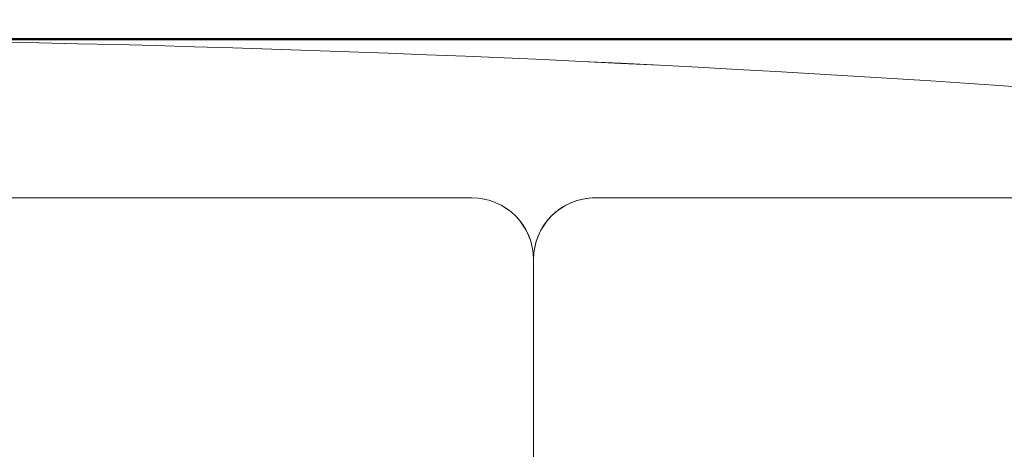
# Model space of a CAD drawing. Units: inches. Extents: x -466983 to 1020, y 324 to 318697.
# Tile 83 of 97: x 650.41 to 662.97, y 948.71 to 954.19. Entities that reach past the tile are written whole.
import ezdxf

# ---------------------------------------------------------------- set-up
doc = ezdxf.new("R2010")
doc.units = ezdxf.units.IN
doc.header["$MEASUREMENT"] = 0
for name, color, linetype, lineweight in [('A-FLOR-PATT', 252, 'Continuous', 13), ('A-FURN', 8, 'Continuous', 18), ('A-WALL', 7, 'Continuous', 50)]:
    doc.layers.add(name, color=color, linetype=linetype, lineweight=lineweight)

# ---------------------------------------------------------------- blocks, each defined once
blk = doc.blocks.new('L Shaped Sofa')
at = {"ltscale": 2}
for p, q in [((2394.712, 728.35), (2394.712, 734.219)), ((2393.28, 726.917), (2377.232, 726.917)), ((2430.914, 726.917), (2396.145, 726.917)), ((2475.263, 723.229), (2377.232, 723.229))]:
    blk.add_line(p, q, dxfattribs=at)
for centre, radius, start, end in [((2393.28, 728.35), 1.433, 270, 0), ((2396.145, 728.35), 1.433, 180, 270), ((2416.36, 1205.029), 481.82, 262.88673, 276.63201)]:
    blk.add_arc(centre, radius, start, end, dxfattribs=at)

msp = doc.modelspace()

# ---------------------------------------------------------------- hatches: boundary and pattern name
at = {"layer": 'A-FLOR-PATT', "transparency": 33554572}
h = msp.add_hatch(dxfattribs=at)
h.set_pattern_fill('ANSI37', color=256, scale=30)
h.set_pattern_definition([(45, (-1212.4137, -290.035), (-2.6516504, 2.6516504), []), (135, (-1212.4137, -290.035), (-2.6516504, -2.6516504), [])])
h.paths.add_polyline_path([(901.806, 1075.938), (900.614, 1075.938), (900.614, 1065.386), (899.391, 1065.386), (898.091, 1065.386), (892.836, 1058.71, -0.258377), (892.188, 1058.351), (879.985, 1058.351, -0.20177), (879.438, 1058.581), (874.081, 1065.386), (872.781, 1065.386), (871.558, 1065.386), (871.558, 1075.938), (813.806, 1075.938), (813.806, 1044.792), (832.395, 1044.792, -0.394795), (848.66, 1028.536), (848.66, 1009.938), (901.806, 1009.938), (901.806, 1015.938), (901.306, 1015.938), (871.306, 1015.938), (871.306, 1017.25), (871.334, 1017.25, -0.401453), (901.306, 1045.938), (901.806, 1045.938)])
edge = h.paths.add_edge_path(flags=16)
edge.add_line((847.773, 1068.949), (847.773, 1073.709))
edge.add_arc((849.227, 1073.709), 1.454, 90, 180, ccw=False)
edge.add_line((849.227, 1075.163), (864.492, 1075.163))
edge.add_arc((864.492, 1073.709), 1.454, 0, 90, ccw=False)
edge.add_line((865.946, 1073.709), (865.946, 1069.004))
edge.add_arc((832.645, 1068.976), 33.301, -20.6123, 0.0472, ccw=False)
edge.add_ellipse((856.859, 1058.48), major_axis=(0, 10.213), ratio=0.685919, start_angle=100.0088, end_angle=259.9912, ccw=False)
edge.add_arc((881.074, 1068.976), 33.301, 180.0472, 200.6123, ccw=False)
h.paths.add_polyline_path([(853.146, 1066.482), (853.146, 1066.453), (853.146, 1066.453, 0.433107), (852.917, 1066.685), (852.917, 1066.453), (853.146, 1066.453), (853.146, 1066.482), (853.088, 1066.612, 0.697939), (852.7, 1066.453), (852.7, 1066.453), (852.7, 1066.482), (852.917, 1067.001), (852.917, 1066.685, -0.396254)], flags=0)
h.paths.add_polyline_path([(861.019, 1066.482), (861.019, 1066.453), (861.019, 1066.453, 0.416404), (860.802, 1066.685), (860.802, 1066.453), (861.019, 1066.453), (861.019, 1066.482), (860.967, 1066.605, 0.713344), (860.573, 1066.453), (860.573, 1066.453), (860.573, 1066.482), (860.802, 1067.001), (860.802, 1066.685, -0.379973)], flags=0)
edge = h.paths.add_edge_path(flags=0)
edge.add_spline(control_points=[(861.13, 1065.785), (861.466, 1065.248), (861.613, 1065.016), (861.983, 1064.374), (862.192, 1063.944), (862.561, 1063.039), (862.721, 1062.563), (862.987, 1061.578), (863.092, 1061.069), (863.245, 1060.031), (863.293, 1059.503), (863.329, 1058.441), (863.318, 1057.908), (863.237, 1056.852), (863.166, 1056.329), (862.97, 1055.308), (862.843, 1054.81), (862.537, 1053.852), (862.357, 1053.393), (861.951, 1052.525), (861.725, 1052.117), (861.233, 1051.362), (860.967, 1051.016), (860.405, 1050.395), (860.108, 1050.12), (859.494, 1049.646), (859.176, 1049.448), (858.528, 1049.13), (858.197, 1049.011), (857.531, 1048.852), (857.196, 1048.812), (856.525, 1048.812), (856.189, 1048.852), (855.524, 1049.01), (855.193, 1049.129), (854.545, 1049.447), (854.227, 1049.645), (853.612, 1050.118), (853.316, 1050.393), (852.753, 1051.014), (852.487, 1051.36), (851.995, 1052.114), (851.769, 1052.523), (851.363, 1053.39), (851.183, 1053.85), (850.877, 1054.807), (850.75, 1055.305), (850.553, 1056.326), (850.483, 1056.849), (850.401, 1057.905), (850.39, 1058.438), (850.426, 1059.5), (850.473, 1060.028), (850.626, 1061.066), (850.732, 1061.575), (850.997, 1062.561), (851.157, 1063.036), (851.525, 1063.942), (851.734, 1064.371), (852.106, 1065.016), (852.254, 1065.25), (852.608, 1065.733)], knot_values=[3.915332, 3.915332, 3.915332, 3.915332, 4.013468, 4.013468, 4.175532, 4.175532, 4.337596, 4.337596, 4.49966, 4.49966, 4.661724, 4.661724, 4.823788, 4.823788, 4.985852, 4.985852, 5.147916, 5.147916, 5.30998, 5.30998, 5.472044, 5.472044, 5.634109, 5.634109, 5.796173, 5.796173, 5.958237, 5.958237, 6.120301, 6.120301, 6.282365, 6.282365, 6.444429, 6.444429, 6.606493, 6.606493, 6.768557, 6.768557, 6.930621, 6.930621, 7.092685, 7.092685, 7.254749, 7.254749, 7.416813, 7.416813, 7.578878, 7.578878, 7.740942, 7.740942, 7.903006, 7.903006, 8.06507, 8.06507, 8.227134, 8.227134, 8.389198, 8.389198, 8.551262, 8.551262, 8.65037, 8.65037, 8.65037, 8.65037], degree=3, periodic=0)
edge.add_line((852.642, 1065.785), (861.13, 1065.785))
edge = h.paths.add_edge_path(flags=0)
edge.add_ellipse((856.85, 1057.743), major_axis=(0, 7.792), ratio=0.687861, start_angle=0, end_angle=360)
h.paths.add_polyline_path([(848.863, 1069.389), (848.863, 1073.96, -0.414214), (849.954, 1075.051), (863.765, 1075.051, -0.414214), (864.856, 1073.96), (864.856, 1069.389, -0.388936), (864.524, 1069.027, -0.043561), (849.195, 1069.027, -0.388936)], flags=0)
h.paths.add_polyline_path([(853.101, 1068.112, -1), (852.677, 1068.112, -1)], flags=0)
edge = h.paths.add_edge_path(flags=0)
edge.add_ellipse((856.859, 1057.338), major_axis=(0, 2.207), ratio=0.657164, start_angle=0, end_angle=360)
h.paths.add_polyline_path([(861.041, 1068.112, -1), (860.618, 1068.112, -1)], flags=0)
edge = h.paths.add_edge_path()
edge.add_line((573.954, 1057.341), (573.954, 1075.938))
edge.add_line((573.954, 1075.938), (558.731, 1075.938))
edge.add_line((558.731, 1075.938), (558.731, 1065.386))
edge.add_line((558.731, 1065.386), (557.507, 1065.386))
edge.add_line((557.507, 1065.386), (556.207, 1065.386))
edge.add_line((556.207, 1065.386), (550.952, 1058.71))
edge.add_arc((550.304, 1059.116), 0.765, 270, 327.9483, ccw=False)
edge.add_line((550.304, 1058.351), (538.101, 1058.351))
edge.add_arc((538.101, 1059.116), 0.765, 224.3704, 270, ccw=False)
edge.add_line((537.555, 1058.581), (532.198, 1065.386))
edge.add_line((532.198, 1065.386), (530.898, 1065.386))
edge.add_line((530.898, 1065.386), (529.674, 1065.386))
edge.add_line((529.674, 1065.386), (529.674, 1075.938))
edge.add_line((529.674, 1075.938), (520.806, 1075.938))
edge.add_line((520.806, 1075.938), (520.806, 1045.938))
edge.add_line((520.806, 1045.938), (521.306, 1045.938))
edge.add_arc((521.306, 1015.938), 30, 2.5075, 90, ccw=False)
edge.add_line((551.277, 1017.25), (551.306, 1017.25))
edge.add_line((551.306, 1017.25), (551.306, 1015.938))
edge.add_line((551.306, 1015.938), (520.806, 1015.938))
edge.add_line((520.806, 1015.938), (520.806, 1009.938))
edge.add_line((520.806, 1009.938), (559.191, 1010.402))
edge.add_arc((559.191, 1011.856), 1.454, 180, 270, ccw=False)
edge.add_line((557.737, 1011.856), (557.737, 1016.561))
edge.add_arc((591.039, 1016.589), 33.301, 159.3877, 180.0472, ccw=False)
edge.add_ellipse((566.824, 1027.085), major_axis=(0, 10.213), ratio=0.685919, start_angle=280.0088, end_angle=439.9912, ccw=False)
edge.add_arc((542.609, 1016.589), 33.301, 0.0472, 20.6123, ccw=False)
edge.add_line((575.91, 1016.616), (575.91, 1011.856))
edge.add_arc((574.456, 1011.856), 1.454, -90, 0, ccw=False)
edge.add_line((574.456, 1010.402), (608.806, 1009.938))
edge.add_line((608.806, 1009.938), (608.806, 1041.086))
edge.add_line((608.806, 1041.086), (590.218, 1041.086))
edge.add_arc((590.775, 1057.907), 16.831, 181.9277, 268.1032, ccw=False)
edge = h.paths.add_edge_path()
edge.add_ellipse((494.244, 583.62), major_axis=(0, 10.213), ratio=0.685919, start_angle=280.0088, end_angle=439.9912, ccw=False)
edge.add_arc((470.03, 573.124), 33.301, 0.0472, 20.6123, ccw=False)
edge.add_line((503.331, 573.152), (503.331, 568.392))
edge.add_arc((501.877, 568.392), 1.454, -90, 0, ccw=False)
edge.add_line((501.877, 566.938), (539.806, 566.938))
edge.add_line((539.806, 566.938), (539.806, 572.938))
edge.add_line((539.806, 572.938), (539.306, 572.938))
edge.add_line((539.306, 572.938), (509.306, 572.938))
edge.add_line((509.306, 572.938), (509.306, 574.25))
edge.add_line((509.306, 574.25), (509.334, 574.25))
edge.add_arc((539.306, 572.938), 30, 90, 177.4925, ccw=False)
edge.add_line((539.306, 602.938), (539.806, 602.938))
edge.add_line((539.806, 602.938), (539.806, 626.938))
edge.add_line((539.806, 626.938), (531.772, 626.938))
edge.add_line((531.772, 626.938), (531.772, 616.386))
edge.add_line((531.772, 616.386), (530.548, 616.386))
edge.add_line((530.548, 616.386), (529.249, 616.386))
edge.add_line((529.249, 616.386), (523.711, 609.351))
edge.add_line((523.711, 609.351), (510.777, 609.351))
edge.add_line((510.777, 609.351), (505.239, 616.386))
edge.add_line((505.239, 616.386), (503.939, 616.386))
edge.add_line((503.939, 616.386), (502.715, 616.386))
edge.add_line((502.715, 616.386), (502.715, 626.938))
edge.add_line((502.715, 626.938), (481.698, 626.938))
edge.add_line((481.698, 626.938), (481.698, 610.995))
edge.add_arc((467.27, 611.473), 14.436, 271.9277, 358.1032, ccw=False)
edge.add_line((467.756, 597.045), (451.806, 597.045))
edge.add_line((451.806, 597.045), (451.806, 584.404))
edge.add_line((451.806, 584.404), (451.806, 566.938))
edge.add_line((451.806, 566.938), (486.612, 566.938))
edge.add_arc((486.612, 568.392), 1.454, 180, 270, ccw=False)
edge.add_line((485.158, 568.392), (485.158, 573.097))
edge.add_arc((518.459, 573.124), 33.301, 159.3877, 180.0472, ccw=False)
h.paths.add_polyline_path([(836.261, 1020.733), (879.89, 1020.733), (879.89, 1039.39), (836.261, 1039.39)], flags=25)
h.paths.add_polyline_path([(549.985, 1036.749), (593.614, 1036.749), (593.614, 1055.407), (549.985, 1055.407)], flags=24)
h.paths.add_polyline_path([(475.123, 595.596), (518.752, 595.596), (518.752, 614.253), (475.123, 614.253)], flags=24)
h = msp.add_hatch(dxfattribs=at)
h.set_pattern_fill('ANSI37', color=256, scale=20)
h.set_pattern_definition([(45, (-1212.4137, -290.035), (-1.767767, 1.767767), []), (135, (-1212.4137, -290.035), (-1.767767, -1.767767), [])])
h.paths.add_polyline_path([(809.806, 870.938), (809.806, 888.152), (806.998, 888.152), (802.662, 888.152), (789.383, 888.152), (786.285, 888.152, -0.414214), (785.499, 888.937), (785.499, 900.196), (785.499, 908.47, -0.414214), (786.808, 909.779, -0.414214), (785.499, 911.088), (785.499, 929.101, -0.414214), (786.808, 930.411, -0.414214), (785.499, 931.72), (785.499, 931.904, -0.414214), (784.19, 930.595), (766.722, 930.595, -0.412359), (765.413, 931.896, -0.413741), (764.115, 930.578), (744.578, 930.422, -0.416556), (743.786, 931.207), (743.786, 933.515), (742.215, 933.515), (742.215, 952.024, -0.001344), (743.786, 952.2), (743.786, 953.938), (678.592, 953.938), (678.592, 951.131), (678.592, 946.794), (678.592, 933.515), (678.592, 930.417, -0.414214), (677.806, 929.631), (666.548, 929.631), (658.274, 929.631, -0.414214), (656.965, 930.94, -0.414214), (655.656, 929.631), (637.642, 929.631, -0.414214), (636.333, 930.94, -0.414214), (635.024, 929.631), (634.839, 929.631, -0.414214), (636.149, 928.322), (636.149, 910.854, -0.412359), (634.848, 909.545, -0.413741), (636.165, 908.247), (636.321, 888.71, -0.416556), (635.536, 887.918), (633.228, 887.918), (633.228, 886.347), (614.719, 886.347, -0.001344), (614.544, 887.918), (612.806, 887.918), (612.806, 834.938), (612.806, 752.938), (612.806, 748.938), (612.806, 697.938), (654.806, 697.938), (654.806, 701.938), (715.806, 701.938), (715.806, 737.435), (774.292, 737.435), (774.292, 795.938), (809.806, 795.938)])
h.paths.add_polyline_path([(679.276, 849.576, 0.102523), (682.148, 849.261, -0.080461), (694.543, 849.773, -0.283899), (694.482, 849.008, 0.136605), (694.407, 848.81, -0.030441), (694.543, 846.893), (694.543, 842.62), (694.543, 838.347, -0.028219), (694.425, 836.568), (694.425, 836.568, 0.196187), (694.446, 836.271, -0.302897), (694.543, 835.467, -0.080461), (682.148, 835.979, 0.102523), (679.276, 835.664, -0.58611), (678.646, 836.017), (678.646, 849.223, -0.58611)], flags=16)
h.paths.add_polyline_path([(679.517, 848.651, 0.699597), (679.476, 848.634, 1.20716), (679.194, 848.742, 0.010621)], flags=0)
h.paths.add_polyline_path([(679.492, 836.561, -0.013798), (679.918, 836.659, -0.071703), (682.853, 837.143, -0.165743), (682.166, 839.101), (682.166, 842.609), (682.166, 846.06, -0.240616), (683.473, 848.677, -0.068263), (693.929, 849.008), (693.788, 848.708), (693.788, 849.023, 0.067332), (683.473, 848.677, 0.240616), (682.166, 846.06), (682.166, 842.609), (682.166, 839.101, 0.23459), (683.461, 836.551, 0.068093), (693.788, 836.195), (693.788, 836.51), (693.93, 836.21, -0.077215), (682.242, 836.782, 0.086627), (679.528, 836.57, -0.628402), (679.503, 836.573), (679.503, 836.607, 0.910458)], flags=0)
h.paths.add_polyline_path([(679.476, 848.636), (679.207, 848.647), (679.207, 836.572, 0.913566), (679.365, 836.586), (679.476, 836.582)], flags=0)
h.paths.add_polyline_path([(679.276, 829.86, 0.102523), (682.148, 829.546, -0.080461), (694.543, 830.057, -0.283899), (694.482, 829.293, 0.136605), (694.407, 829.095, -0.030441), (694.543, 827.178), (694.543, 822.904), (694.543, 818.631, -0.028219), (694.425, 816.853), (694.425, 816.853, 0.196187), (694.446, 816.556, -0.302897), (694.543, 815.752, -0.080461), (682.148, 816.263, 0.102523), (679.276, 815.949, -0.58611), (678.646, 816.302), (678.646, 829.507, -0.58611)], flags=16)
h.paths.add_polyline_path([(679.517, 828.936, 0.699597), (679.476, 828.919, 1.20716), (679.194, 829.027, 0.010621)], flags=0)
h.paths.add_polyline_path([(679.492, 816.846, -0.013798), (679.918, 816.944, -0.071703), (682.853, 817.428, -0.165743), (682.166, 819.385), (682.166, 822.894), (682.166, 826.345, -0.240616), (683.473, 828.961, -0.068263), (693.929, 829.293), (693.788, 828.993), (693.788, 829.308, 0.067332), (683.473, 828.961, 0.240616), (682.166, 826.345), (682.166, 822.894), (682.166, 819.385, 0.23459), (683.461, 816.836, 0.068093), (693.788, 816.48), (693.788, 816.795), (693.93, 816.495, -0.077215), (682.242, 817.066, 0.086627), (679.528, 816.855, -0.628402), (679.503, 816.858), (679.503, 816.892, 0.910458)], flags=0)
h.paths.add_polyline_path([(679.476, 828.921), (679.207, 828.932), (679.207, 816.857, 0.913566), (679.365, 816.871), (679.476, 816.867)], flags=0)
h.paths.add_polyline_path([(679.276, 810.145, 0.102523), (682.148, 809.83, -0.080461), (694.543, 810.342, -0.3023), (694.447, 809.539, 0.10023), (694.406, 809.388, -0.03057), (694.543, 807.462), (694.543, 803.189), (694.543, 798.916, -0.03057), (694.406, 796.991, 0.10023), (694.447, 796.839, -0.3023), (694.543, 796.036, -0.080461), (682.148, 796.548, 0.102523), (679.276, 796.233, -0.58611), (678.646, 796.586), (678.646, 809.792, -0.58611)], flags=16)
h.paths.add_polyline_path([(679.517, 809.242, 0.699597), (679.476, 809.224, 1.20716), (679.194, 809.332, 0.010621)], flags=0)
h.paths.add_polyline_path([(679.492, 797.151, -0.013798), (679.918, 797.25, -0.071703), (682.853, 797.734, -0.165743), (682.166, 799.691), (682.166, 803.2), (682.166, 806.65, -0.239349), (683.461, 809.258, -0.072465), (694.447, 809.541, 0.197932), (694.425, 809.241), (693.788, 809.299), (693.788, 809.614, 0.068093), (683.461, 809.258, 0.239349), (682.166, 806.65), (682.166, 803.2), (682.166, 799.691, 0.235854), (683.473, 797.132, 0.067332), (693.788, 796.786), (693.788, 797.101), (694.425, 797.159, 0.197932), (694.447, 796.859, -0.080419), (682.156, 797.379, 0.083867), (679.528, 797.16, -0.628402), (679.503, 797.164), (679.503, 797.197, 0.910458)], flags=0)
h.paths.add_polyline_path([(679.207, 809.237), (679.207, 797.162, 0.913566), (679.365, 797.176), (679.476, 797.173), (679.476, 809.227)], flags=0)
h.paths.add_polyline_path([(695.364, 853.299), (728.223, 853.299), (728.223, 771.152), (695.364, 771.152)], flags=16)
h.paths.add_polyline_path([(696.021, 852.642), (727.566, 852.642), (727.566, 771.809), (696.021, 771.809)], flags=0)
h.paths.add_polyline_path([(679.276, 788.787, 0.102523), (682.148, 788.472, -0.080461), (694.543, 788.984, -0.3023), (694.447, 788.181, 0.10023), (694.406, 788.03, -0.03057), (694.543, 786.104), (694.543, 781.831), (694.543, 777.558, -0.03057), (694.406, 775.632, 0.10023), (694.447, 775.481, -0.3023), (694.543, 774.678, -0.080461), (682.148, 775.19, 0.102523), (679.276, 774.875, -0.58611), (678.646, 775.228), (678.646, 788.434, -0.58611)], flags=16)
h.paths.add_polyline_path([(679.517, 787.883, 0.699597), (679.476, 787.866, 1.20716), (679.194, 787.974, 0.010621)], flags=0)
h.paths.add_polyline_path([(679.492, 775.793, -0.013798), (679.918, 775.891, -0.071703), (682.853, 776.375, -0.165743), (682.166, 778.333), (682.166, 781.841), (682.166, 785.292, -0.239349), (683.461, 787.899, -0.072465), (694.447, 788.182, 0.197932), (694.425, 787.882), (693.788, 787.94), (693.788, 788.255, 0.068093), (683.461, 787.899, 0.239349), (682.166, 785.292), (682.166, 781.841), (682.166, 778.333, 0.235854), (683.473, 775.774, 0.067332), (693.788, 775.428), (693.788, 775.742), (694.425, 775.8, 0.197932), (694.447, 775.5, -0.080419), (682.156, 776.021, 0.083867), (679.528, 775.802, -0.628402), (679.503, 775.805), (679.503, 775.839, 0.910458)], flags=0)
h.paths.add_polyline_path([(679.207, 787.879), (679.207, 775.804, 0.913566), (679.365, 775.818), (679.476, 775.814), (679.476, 787.868)], flags=0)
h.paths.add_polyline_path([(704.641, 854.12, -0.080461), (705.153, 866.516, 0.102523), (704.838, 869.387, -0.58611), (705.191, 870.017), (718.397, 870.017, -0.58611), (718.75, 869.387, 0.102523), (718.435, 866.516, -0.080461), (718.946, 854.12, -0.3023), (718.144, 854.217, 0.10023), (717.992, 854.257, -0.03057), (716.067, 854.12), (711.794, 854.12), (707.521, 854.12, -0.03057), (705.595, 854.257, 0.10023), (705.444, 854.217, -0.3023)], flags=16)
h.paths.add_polyline_path([(717.846, 869.146, 0.699597), (717.829, 869.187, 1.20716), (717.937, 869.47, 0.010621)], flags=0)
h.paths.add_polyline_path([(705.463, 854.216, -0.080419), (705.984, 866.507, 0.083867), (705.765, 869.135, -0.628402), (705.768, 869.16), (705.802, 869.16, 0.910458), (705.756, 869.171, -0.013798), (705.854, 868.745, -0.071703), (706.338, 865.81, -0.165743), (708.295, 866.497), (711.804, 866.497), (715.255, 866.497, -0.239349), (717.862, 865.202, -0.072465), (718.145, 854.216, 0.197932), (717.845, 854.238), (717.903, 854.876), (718.218, 854.876, 0.068093), (717.862, 865.202, 0.239349), (715.255, 866.497), (711.804, 866.497), (708.295, 866.497, 0.235854), (705.737, 865.19, 0.067332), (705.391, 854.876), (705.705, 854.876), (705.763, 854.238, 0.197932)], flags=16)
h.paths.add_polyline_path([(705.766, 869.456, 0.913566), (705.781, 869.299), (705.777, 869.187), (717.831, 869.187), (717.842, 869.456)], flags=0)
h.paths.add_polyline_path([(729.045, 842.62), (729.045, 846.893, -0.03057), (729.182, 848.818, 0.10023), (729.141, 848.97, -0.3023), (729.045, 849.773, -0.080461), (741.44, 849.261, 0.102523), (744.311, 849.576, -0.58611), (744.942, 849.223), (744.942, 836.017, -0.58611), (744.311, 835.664, 0.102523), (741.44, 835.979, -0.080461), (729.045, 835.467, -0.3023), (729.141, 836.27, 0.10023), (729.182, 836.421, -0.03057), (729.045, 838.347)], flags=16)
h.paths.add_polyline_path([(744.111, 836.585, 1.20716), (744.394, 836.477, 0.010621), (744.07, 836.567, 0.699597)], flags=0)
h.paths.add_polyline_path([(729.141, 836.268, 0.197932), (729.162, 836.568), (729.8, 836.51), (729.8, 836.195, 0.068093), (740.126, 836.551, 0.239349), (741.421, 839.159), (741.421, 842.609), (741.421, 846.118, 0.235854), (740.114, 848.677, 0.067332), (729.8, 849.023), (729.8, 848.708), (729.162, 848.65, 0.197932), (729.141, 848.95, -0.080419), (741.432, 848.43, 0.083867), (744.059, 848.649, -0.628402), (744.085, 848.645), (744.085, 848.612, 0.910458), (744.095, 848.658, -0.013798), (743.67, 848.559, -0.071703), (740.734, 848.075, -0.165743), (741.421, 846.118), (741.421, 842.609), (741.421, 839.159, -0.239349), (740.126, 836.551, -0.072465)], flags=0)
h.paths.add_polyline_path([(729.045, 830.057, -0.080461), (741.44, 829.546, 0.102523), (744.311, 829.86, -0.58611), (744.942, 829.507), (744.942, 816.302, -0.58611), (744.311, 815.949, 0.102523), (741.44, 816.263, -0.080461), (729.045, 815.752, -0.3023), (729.141, 816.554, 0.10023), (729.182, 816.706, -0.03057), (729.045, 818.631), (729.045, 822.904), (729.045, 827.178, -0.03057), (729.182, 829.103, 0.10023), (729.141, 829.255, -0.3023)], flags=16)
h.paths.add_polyline_path([(744.111, 816.869, 1.20716), (744.394, 816.761, 0.010621), (744.07, 816.852, 0.699597)], flags=0)
h.paths.add_polyline_path([(729.141, 829.235, -0.080419), (741.432, 828.714, 0.083867), (744.059, 828.933, -0.628402), (744.085, 828.93), (744.085, 828.896, 0.910458), (744.095, 828.943, -0.013798), (743.67, 828.844, -0.071703), (740.734, 828.36, -0.165743), (741.421, 826.403), (741.421, 822.894), (741.421, 819.443, -0.239349), (740.126, 816.836, -0.072465), (729.141, 816.553, 0.197932), (729.162, 816.853), (729.8, 816.795), (729.8, 816.48, 0.068093), (740.126, 816.836, 0.239349), (741.421, 819.443), (741.421, 822.894), (741.421, 826.403, 0.235854), (740.114, 828.961, 0.067332), (729.8, 829.308), (729.8, 828.993), (729.162, 828.935, 0.197932)], flags=16)
h.paths.add_polyline_path([(729.045, 810.342, -0.080461), (741.44, 809.83, 0.102523), (744.311, 810.145, -0.58611), (744.942, 809.792), (744.942, 796.586, -0.58611), (744.311, 796.233, 0.102523), (741.44, 796.548, -0.080461), (729.045, 796.036, -0.283899), (729.105, 796.801, 0.136605), (729.181, 796.999, -0.030441), (729.045, 798.916), (729.045, 803.189), (729.045, 807.462, -0.028219), (729.163, 809.241), (729.162, 809.241, 0.196187), (729.142, 809.538, -0.302897)], flags=16)
h.paths.add_polyline_path([(744.111, 797.175, 1.20716), (744.394, 797.067, 0.010621), (744.07, 797.158, 0.699597)], flags=0)
h.paths.add_polyline_path([(741.345, 809.027, 0.086627), (744.059, 809.239, -0.628402), (744.085, 809.235), (744.085, 809.202, 0.910458), (744.095, 809.248, -0.013798), (743.67, 809.15, -0.071703), (740.734, 808.666, -0.165743), (741.421, 806.708), (741.421, 803.2), (741.421, 799.749, -0.240616), (740.114, 797.132, -0.068263), (729.658, 796.801), (729.8, 797.101), (729.8, 796.786, 0.067332), (740.114, 797.132, 0.240616), (741.421, 799.749), (741.421, 803.2), (741.421, 806.708, 0.23459), (740.126, 809.258, 0.068093), (729.8, 809.614), (729.8, 809.299), (729.658, 809.599, -0.077215)], flags=0)
h.paths.add_polyline_path([(704.641, 770.33, -0.283899), (705.405, 770.27, 0.136605), (705.603, 770.194, -0.030441), (707.521, 770.33), (711.794, 770.33), (716.067, 770.33, -0.028219), (717.845, 770.212), (717.845, 770.213, 0.196187), (718.143, 770.233, -0.302897), (718.946, 770.33, -0.080461), (718.435, 757.935, 0.102523), (718.75, 755.064, -0.58611), (718.397, 754.433), (705.191, 754.433, -0.58611), (704.838, 755.064, 0.102523), (705.153, 757.935, -0.080461)], flags=16)
h.paths.add_polyline_path([(705.762, 755.305, 0.699597), (705.779, 755.264, 1.20716), (705.671, 754.981, 0.010621)], flags=0)
h.paths.add_polyline_path([(705.405, 769.717), (705.705, 769.575), (705.391, 769.575, 0.067332), (705.737, 759.261, 0.240616), (708.353, 757.954), (711.804, 757.954), (715.313, 757.954, 0.23459), (717.862, 759.249, 0.068093), (718.218, 769.575), (717.903, 769.575), (718.203, 769.717, -0.077215), (717.632, 758.03, 0.086627), (717.843, 755.316, -0.628402), (717.84, 755.29), (717.806, 755.29, 0.910458), (717.853, 755.28, -0.013798), (717.754, 755.705, -0.071703), (717.27, 758.641, -0.165743), (715.313, 757.954), (711.804, 757.954), (708.353, 757.954, -0.240616), (705.737, 759.261, -0.068263)], flags=0)
h.paths.add_polyline_path([(729.045, 788.984, -0.080461), (741.44, 788.472, 0.102523), (744.311, 788.787, -0.58611), (744.942, 788.434), (744.942, 775.228, -0.58611), (744.311, 774.875, 0.102523), (741.44, 775.19, -0.080461), (729.045, 774.678, -0.283899), (729.105, 775.443, 0.136605), (729.181, 775.64, -0.030441), (729.045, 777.558), (729.045, 781.831), (729.045, 786.104, -0.028219), (729.163, 787.882), (729.162, 787.882, 0.196187), (729.142, 788.18, -0.302897)], flags=16)
h.paths.add_polyline_path([(744.111, 775.817, 1.20716), (744.394, 775.709, 0.010621), (744.07, 775.799, 0.699597)], flags=0)
h.paths.add_polyline_path([(741.345, 787.669, 0.086627), (744.059, 787.881, -0.628402), (744.085, 787.877), (744.085, 787.844, 0.910458), (744.095, 787.89, -0.013798), (743.67, 787.791, -0.071703), (740.734, 787.307, -0.165743), (741.421, 785.35), (741.421, 781.841), (741.421, 778.39, -0.240616), (740.114, 775.774, -0.068263), (729.658, 775.443), (729.8, 775.742), (729.8, 775.428, 0.067332), (740.114, 775.774, 0.240616), (741.421, 778.39), (741.421, 781.841), (741.421, 785.35, 0.23459), (740.126, 787.899, 0.068093), (729.8, 788.255), (729.8, 787.94), (729.658, 788.241, -0.077215)], flags=0)
h.paths.add_polyline_path([(744.111, 848.636), (744.111, 836.582), (744.381, 836.572), (744.381, 848.647, 0.913566), (744.223, 848.633)], flags=0)
h.paths.add_polyline_path([(744.223, 828.917), (744.111, 828.921), (744.111, 816.867), (744.381, 816.857), (744.381, 828.932, 0.913566)], flags=0)
h.paths.add_polyline_path([(717.831, 755.264), (705.777, 755.264), (705.766, 754.994), (717.842, 754.994, 0.913566), (717.827, 755.152)], flags=0)
h.paths.add_polyline_path([(744.223, 809.223), (744.111, 809.227), (744.111, 797.173), (744.381, 797.162), (744.381, 809.237, 0.913566)], flags=0)
h.paths.add_polyline_path([(744.111, 787.868), (744.111, 775.814), (744.381, 775.804), (744.381, 787.879, 0.913566), (744.223, 787.865)], flags=0)
h.paths.add_polyline_path([(678.877, 877.123), (737.613, 877.123), (737.613, 899.512), (678.877, 899.512)], flags=24)

# ---------------------------------------------------------------- linework, layer by layer
at = {"layer": 'A-FURN', "ltscale": 2}
for p, q in [((612.806, 953.938), (666.548, 953.938)), ((612.806, 953.938), (666.548, 953.938)), ((612.806, 953.938), (666.548, 953.938)), ((612.806, 953.938), (666.548, 953.938)), ((612.806, 953.938), (666.548, 953.938)), ((612.806, 953.938), (666.548, 953.938)), ((637.118, 951.916), (656.179, 951.916)), ((637.118, 951.916), (656.179, 951.916)), ((637.118, 951.916), (656.179, 951.916)), ((637.118, 951.916), (656.179, 951.916)), ((637.118, 951.916), (656.179, 951.916)), ((637.118, 951.916), (656.179, 951.916)), ((657.75, 951.916), (666.548, 951.916)), ((657.75, 951.916), (666.548, 951.916)), ((657.75, 951.916), (666.548, 951.916)), ((657.75, 951.916), (666.548, 951.916)), ((657.75, 951.916), (666.548, 951.916)), ((657.75, 951.916), (666.548, 951.916)), ((656.965, 951.131), (656.965, 947.913)), ((656.965, 951.131), (656.965, 947.913)), ((656.965, 951.131), (656.965, 947.913)), ((656.965, 951.131), (656.965, 947.913)), ((656.965, 951.131), (656.965, 947.913)), ((656.965, 951.131), (656.965, 947.913))]:
    msp.add_line(p, q, dxfattribs=at)
for centre, radius, start, end in [((645.097, 689.808), 264.141, 82.88673, 96.63201), ((645.097, 689.808), 264.141, 82.88673, 96.63201), ((645.097, 689.808), 264.141, 82.88673, 96.63201), ((645.097, 689.808), 264.141, 82.88673, 96.63201), ((645.097, 689.808), 264.141, 82.88673, 96.63201), ((645.097, 689.808), 264.141, 82.88673, 96.63201), ((656.179, 951.131), 0.785, 0, 90), ((656.179, 951.131), 0.785, 0, 90), ((656.179, 951.131), 0.785, 0, 90), ((656.179, 951.131), 0.785, 0, 90), ((656.179, 951.131), 0.785, 0, 90), ((656.179, 951.131), 0.785, 0, 90), ((657.75, 951.131), 0.785, 90, 180), ((657.75, 951.131), 0.785, 90, 180), ((657.75, 951.131), 0.785, 90, 180), ((657.75, 951.131), 0.785, 90, 180), ((657.75, 951.131), 0.785, 90, 180), ((657.75, 951.131), 0.785, 90, 180)]:
    msp.add_arc(centre, radius, start, end, dxfattribs=at)
at = {"layer": 'A-WALL'}
msp.add_line((612.806, 953.938), (680.592, 953.938), dxfattribs=at)

# ---------------------------------------------------------------- block references
at = {"layer": 'A-FURN', "xscale": 0.5482153745360612, "yscale": 0.5482153745360612, "zscale": 0.5482153745360612, "rotation": 180}
msp.add_blockref('L Shaped Sofa', (1969.783, 1350.423), dxfattribs=at)

doc.saveas('drawing.dxf')
